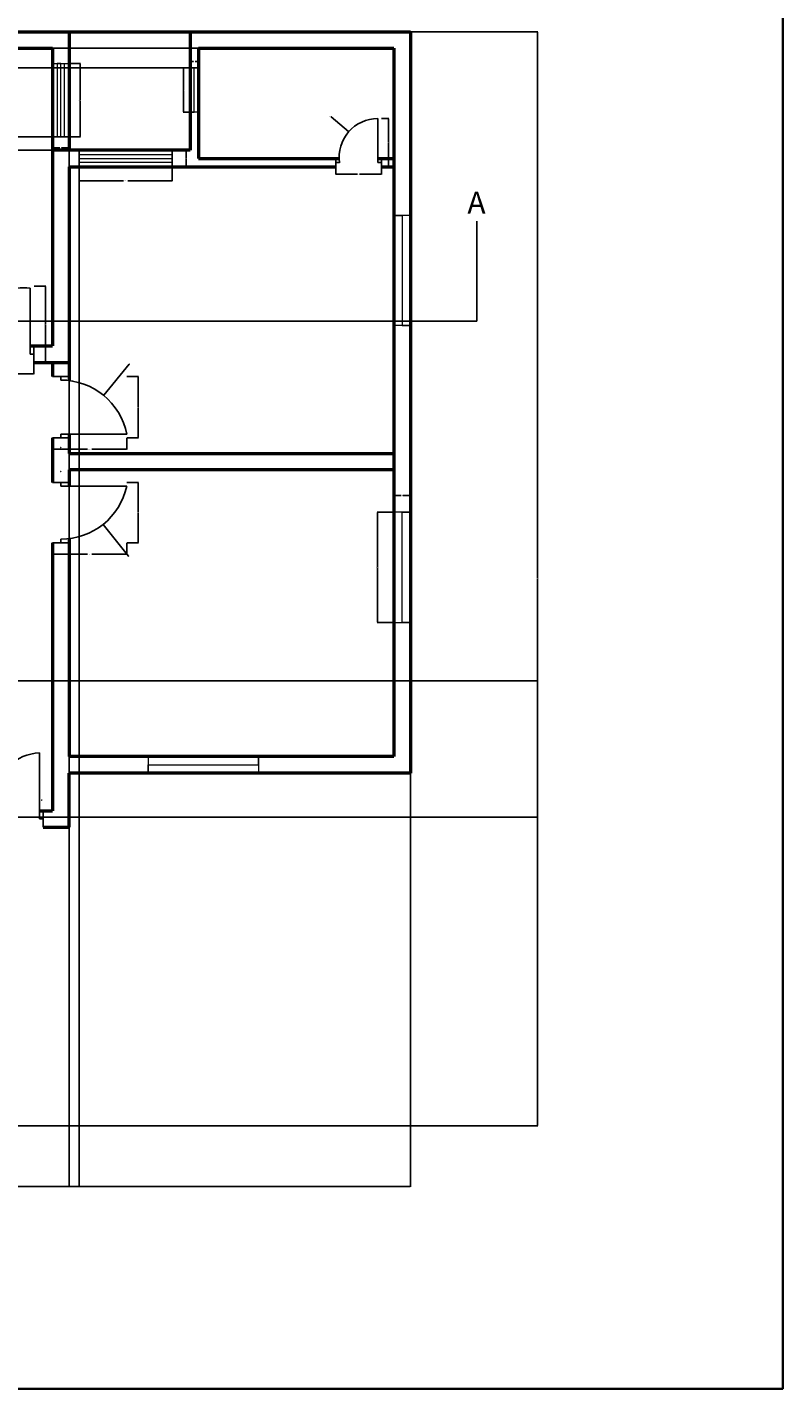
# Model space of a CAD drawing. Units: inches. Extents: x 2215 to 3724, y 1009 to 2124.
# Tile 10 of 11: x 3312 to 3724, y 1009 to 1750. Entities that reach past the tile are written whole.
import ezdxf

# ---------------------------------------------------------------- set-up
doc = ezdxf.new("R2010")
doc.units = ezdxf.units.IN
for name, color, linetype, lineweight in [('A-ANNO-DIMS', 2, 'Continuous', 18), ('A-ANNO-SYMB', 7, 'Continuous', 25), ('A-ANNO-TTLB', 7, 'Continuous', 35), ('A-DOOR', 3, 'Continuous', 25), ('A-GLAZ', 4, 'Continuous', 18), ('A-WALL', 7, 'Continuous', 50)]:
    doc.layers.add(name, color=color, linetype=linetype, lineweight=lineweight)
doc.styles.get("Standard").update_dxf_attribs({"font": 'arial.ttf'})
doc.dimstyles.get("Standard").update_dxf_attribs({"dimtxt": 0.18, "dimasz": 0.18, "dimexe": 0.18, "dimexo": 0.0625, "dimgap": 0.09, "dimtad": 0, "dimtih": 1, "dimtoh": 1, "dimdec": 4, "dimzin": 0, "dimdsep": 46, "dimtxsty": 'Standard', "dimcen": 0.09, "dimadec": 0, "dimazin": 0, "dimtfac": 1, "dimtdec": 4, "dimtofl": 0, "dimtmove": 0, "dimatfit": 3, "dimfxl": 1, "dimtolj": 1, "dimtzin": 0, "dimarcsym": 0})

# ---------------------------------------------------------------- blocks, each defined once
blk = doc.blocks.new('DOOR-BEDROOM-NE')
for p, q in [((0, 33.52), (0, 33.52)), ((0, 33.52), (9, 33.52)), ((9, 33.52), (4.5, 33.52)), ((4.5, 33.52), (4.5, 31.52)), ((0, 0), (9, 0)), ((4.5, 0), (4.5, 2)), ((4.5, 2), (40.5, 2)), ((9, 0), (4.5, 0))]:
    blk.add_line(p, q)
blk.add_arc((4.5, -5.19), 36.71, 11.299, 90)
blk = doc.blocks.new('DOOR-BEDROOM-SE')
for p, q in [((9, 32.82), (0, 32.82)), ((0, 32.82), (4.5, 32.82)), ((4.5, 32.82), (4.5, 30.82)), ((4.5, 30.82), (40.5, 30.82)), ((0, 0), (0, 0)), ((0, 0), (9, 0)), ((4.5, 0), (4.5, 2)), ((9, 0), (4.5, 0))]:
    blk.add_line(p, q)
blk.add_arc((4.5, 38.9), 36.9, 270, 347.35338)
blk = doc.blocks.new('DOOR-ENTRY-PAIR')
for p, q in [((2, 4.5), (2, 40.5)), ((54.26, 4.5), (54.26, 40.5)), ((0, 9), (0, 0)), ((56.26, 9), (56.26, 0)), ((0, 0), (0, 4.5)), ((0, 4.5), (2, 4.5)), ((56.26, 4.5), (54.26, 4.5))]:
    blk.add_line(p, q)
for centre, radius, start, end in [((2, 12.02), 28.48, 11.01665, 90), ((55.55, 14.8), 25.73, 92.87958, 174.07084)]:
    blk.add_arc(centre, radius, start, end)
blk = doc.blocks.new('DOOR-BATH-NE')
for p, q in [((22.84, 2.25), (22.84, 26.25)), ((0, 4.5), (0, 0)), ((0, 0), (0, 2.25)), ((0, 2.25), (2, 2.25)), ((24.84, 2.25), (22.84, 2.25)), ((24.84, 4.5), (24.84, 0)), ((24.84, 0), (24.84, 2.25))]:
    blk.add_line(p, q)
blk.add_arc((22.84, 5.2), 21.05, 90, 188.0713)
blk = doc.blocks.new('DOOR-BEDROOM-N')
for p, q in [((37.14, 4.5), (37.14, 40.5)), ((0, 9), (0, 0)), ((39.14, 9), (39.14, 0)), ((0, 0), (0, 4.5)), ((0, 4.5), (2, 4.5)), ((39.14, 4.5), (37.14, 4.5)), ((39.14, 0), (39.14, 4.5))]:
    blk.add_line(p, q)
blk.add_arc((33.66, 8.74), 31.95, 83.74408, 187.63495)
blk = doc.blocks.new('WIN-60-JAMB-A')
for p, q in [((0, 9), (0, 0)), ((60, 4.5), (60, 9)), ((60, 9), (60, 0)), ((0, 0), (0, 4.5)), ((0, 4.5), (60, 4.5))]:
    blk.add_line(p, q)
blk = doc.blocks.new('WIN-OTS-E-END')
for p, q in [((0, 9), (0, 0)), ((50.62, 4.5), (50.62, 9)), ((50.62, 9), (50.62, 0)), ((50.62, 6.5), (0, 6.5)), ((0, 6.5), (0, 4.5)), ((0, 0), (0, 4.5)), ((0, 4.5), (50.62, 4.5)), ((0, 4.5), (0, 2.5)), ((0, 2.5), (50.62, 2.5)), ((50.62, 4.5), (50.62, 6.5)), ((50.62, 0), (50.62, 4.5))]:
    blk.add_line(p, q)
blk = doc.blocks.new('WIN-60-JAMB-B')
for p, q in [((9, 60), (0, 60)), ((0, 60), (4.5, 60)), ((4.5, 60), (4.5, 0)), ((4.5, 0), (0, 0)), ((0, 0), (9, 0))]:
    blk.add_line(p, q)
blk = doc.blocks.new('WIN-OTS-E-SIDE')
for p, q in [((0, 39.84), (9, 39.84)), ((3.5, 39.84), (2.5, 39.84)), ((2.5, 39.84), (2.5, 0)), ((4.5, 39.84), (3.5, 39.84)), ((4.5, 0), (4.5, 39.84)), ((6.5, 0), (6.5, 39.84)), ((9, 0), (0, 0)), ((0, 0), (4.5, 0)), ((2.5, 0), (4.5, 0)), ((4.5, 0), (6.5, 0))]:
    blk.add_line(p, q)
blk = doc.blocks.new('VENT-24-NE')
for p, q in [((0, 24), (4.5, 24)), ((4.5, 24), (2.25, 24)), ((2.25, 24), (2.25, 0)), ((2.25, 0), (0, 0)), ((0, 0), (4.5, 0))]:
    blk.add_line(p, q)
blk = doc.blocks.new('*D33')
at = {"layer": 'A-ANNO-DIMS', "color": 0, "lineweight": -2, "transparency": 16777216}
for p, q in [((3511.68, 1485.98), (3502.56, 1485.98)), ((3502.74, 1485.8), (3502.74, 1456.16)), ((3502.74, 1426.16), (3502.74, 1455.79)), ((3511.68, 1425.98), (3502.56, 1425.98))]:
    blk.add_line(p, q, dxfattribs=at)
at = {"layer": 'A-ANNO-DIMS', "color": 0, "transparency": 16777216}
for points in [[(3502.71, 1485.8), (3502.77, 1485.8), (3502.74, 1485.98)], [(3502.71, 1426.16), (3502.77, 1426.16), (3502.74, 1425.98)]]:
    blk.add_solid(points, dxfattribs=at)
at = {"layer": 'Defpoints', "color": 0, "transparency": 16777216}
for p in [(3511.74, 1485.98), (3502.74, 1425.98), (3511.74, 1425.98)]:
    blk.add_point(p, dxfattribs=at)
at = {"layer": 'A-ANNO-DIMS', "color": 0, "transparency": 16777216, "insert": (3502.74, 1455.98), "char_height": 0.18, "attachment_point": 5}
blk.add_mtext('\\A1;WINDOW 60 TYP.', dxfattribs=at)
blk = doc.blocks.new('*D34')
at = {"layer": 'A-ANNO-DIMS', "color": 0, "lineweight": -2, "transparency": 16777216}
for p, q in [((3511.74, 1486.04), (3511.74, 1495.16)), ((3511.92, 1494.98), (3515.79, 1494.98)), ((3520.56, 1494.98), (3516.7, 1494.98)), ((3520.74, 1486.04), (3520.74, 1495.16))]:
    blk.add_line(p, q, dxfattribs=at)
at = {"layer": 'A-ANNO-DIMS', "color": 0, "transparency": 16777216}
for points in [[(3511.92, 1495.01), (3511.92, 1494.95), (3511.74, 1494.98)], [(3520.56, 1495.01), (3520.56, 1494.95), (3520.74, 1494.98)]]:
    blk.add_solid(points, dxfattribs=at)
at = {"layer": 'Defpoints', "color": 0, "transparency": 16777216}
for p in [(3511.74, 1494.98), (3511.74, 1485.98), (3520.74, 1485.98)]:
    blk.add_point(p, dxfattribs=at)
at = {"layer": 'A-ANNO-DIMS', "color": 0, "transparency": 16777216, "insert": (3516.24, 1494.98), "char_height": 0.18, "attachment_point": 5}
blk.add_mtext('\\A1;9 TYP.', dxfattribs=at)
blk = doc.blocks.new('*D35')
at = {"layer": 'A-ANNO-DIMS', "color": 0, "lineweight": -2, "transparency": 16777216}
for p, q in [((3340.3, 1673.93), (3340.3, 1666.22)), ((3390.92, 1673.93), (3390.92, 1666.22)), ((3340.48, 1666.4), (3364.49, 1666.4)), ((3390.74, 1666.4), (3366.73, 1666.4))]:
    blk.add_line(p, q, dxfattribs=at)
at = {"layer": 'A-ANNO-DIMS', "color": 0, "transparency": 16777216}
for points in [[(3340.48, 1666.43), (3340.48, 1666.37), (3340.3, 1666.4)], [(3390.74, 1666.43), (3390.74, 1666.37), (3390.92, 1666.4)]]:
    blk.add_solid(points, dxfattribs=at)
at = {"layer": 'Defpoints', "color": 0, "transparency": 16777216}
for p in [(3340.3, 1674), (3390.92, 1674), (3390.92, 1666.4)]:
    blk.add_point(p, dxfattribs=at)
at = {"layer": 'A-ANNO-DIMS', "color": 0, "transparency": 16777216, "insert": (3365.61, 1666.4), "char_height": 0.18, "attachment_point": 5}
blk.add_mtext('\\A1;WINDOW 51 TYP.', dxfattribs=at)
blk = doc.blocks.new('*D36')
at = {"layer": 'A-ANNO-DIMS', "color": 0, "lineweight": -2, "transparency": 16777216}
for p, q in [((3390.98, 1683), (3398.69, 1683)), ((3398.51, 1682.82), (3398.51, 1678.68)), ((3398.51, 1674.18), (3398.51, 1678.32)), ((3390.98, 1674), (3398.69, 1674))]:
    blk.add_line(p, q, dxfattribs=at)
at = {"layer": 'A-ANNO-DIMS', "color": 0, "transparency": 16777216}
for points in [[(3398.48, 1682.82), (3398.54, 1682.82), (3398.51, 1683)], [(3398.48, 1674.18), (3398.54, 1674.18), (3398.51, 1674)]]:
    blk.add_solid(points, dxfattribs=at)
at = {"layer": 'Defpoints', "color": 0, "transparency": 16777216}
for p in [(3390.92, 1683), (3398.51, 1683), (3390.92, 1674)]:
    blk.add_point(p, dxfattribs=at)
at = {"layer": 'A-ANNO-DIMS', "color": 0, "transparency": 16777216, "insert": (3398.51, 1678.5), "char_height": 0.18, "attachment_point": 5}
blk.add_mtext('\\A1;9 TYP.', dxfattribs=at)
blk = doc.blocks.new('*D37')
at = {"layer": 'A-ANNO-DIMS', "color": 0, "lineweight": -2, "transparency": 16777216}
for p, q in [((3334.81, 1730.15), (3340.9, 1730.15)), ((3340.72, 1729.97), (3340.72, 1710.41)), ((3340.72, 1690.49), (3340.72, 1710.05)), ((3334.81, 1690.31), (3340.9, 1690.31))]:
    blk.add_line(p, q, dxfattribs=at)
at = {"layer": 'A-ANNO-DIMS', "color": 0, "transparency": 16777216}
for points in [[(3340.69, 1729.97), (3340.75, 1729.97), (3340.72, 1730.15)], [(3340.69, 1690.49), (3340.75, 1690.49), (3340.72, 1690.31)]]:
    blk.add_solid(points, dxfattribs=at)
at = {"layer": 'Defpoints', "color": 0, "transparency": 16777216}
for p in [(3334.74, 1730.15), (3340.72, 1730.15), (3334.74, 1690.31)]:
    blk.add_point(p, dxfattribs=at)
at = {"layer": 'A-ANNO-DIMS', "color": 0, "transparency": 16777216, "insert": (3340.72, 1710.23), "char_height": 0.18, "attachment_point": 5}
blk.add_mtext('\\A1;WINDOW 40 TYP.', dxfattribs=at)
blk = doc.blocks.new('*D38')
at = {"layer": 'A-ANNO-DIMS', "color": 0, "lineweight": -2, "transparency": 16777216}
for p, q in [((3325.74, 1690.25), (3325.74, 1684.15)), ((3334.74, 1690.25), (3334.74, 1684.15)), ((3325.92, 1684.33), (3329.79, 1684.33)), ((3334.56, 1684.33), (3330.7, 1684.33))]:
    blk.add_line(p, q, dxfattribs=at)
at = {"layer": 'A-ANNO-DIMS', "color": 0, "transparency": 16777216}
for points in [[(3325.92, 1684.36), (3325.92, 1684.3), (3325.74, 1684.33)], [(3334.56, 1684.36), (3334.56, 1684.3), (3334.74, 1684.33)]]:
    blk.add_solid(points, dxfattribs=at)
at = {"layer": 'Defpoints', "color": 0, "transparency": 16777216}
for p in [(3325.74, 1690.31), (3334.74, 1690.31), (3334.74, 1684.33)]:
    blk.add_point(p, dxfattribs=at)
at = {"layer": 'A-ANNO-DIMS', "color": 0, "transparency": 16777216, "insert": (3330.24, 1684.33), "char_height": 0.18, "attachment_point": 5}
blk.add_mtext('\\A1;9 TYP.', dxfattribs=at)
blk = doc.blocks.new('*D49')
at = {"layer": 'A-ANNO-DIMS', "color": 0, "lineweight": -2, "transparency": 16777216}
for p, q in [((3400.68, 1727.79), (3396.96, 1727.79)), ((3397.14, 1727.61), (3397.14, 1715.97)), ((3397.14, 1703.97), (3397.14, 1715.61)), ((3400.68, 1703.79), (3396.96, 1703.79))]:
    blk.add_line(p, q, dxfattribs=at)
at = {"layer": 'A-ANNO-DIMS', "color": 0, "transparency": 16777216}
for points in [[(3397.11, 1727.61), (3397.17, 1727.61), (3397.14, 1727.79)], [(3397.11, 1703.97), (3397.17, 1703.97), (3397.14, 1703.79)]]:
    blk.add_solid(points, dxfattribs=at)
at = {"layer": 'Defpoints', "color": 0, "transparency": 16777216}
for p in [(3400.74, 1727.79), (3397.14, 1703.79), (3400.74, 1703.79)]:
    blk.add_point(p, dxfattribs=at)
at = {"layer": 'A-ANNO-DIMS', "color": 0, "transparency": 16777216, "insert": (3397.14, 1715.79), "char_height": 0.18, "attachment_point": 5}
blk.add_mtext('\\A1;VENT 24 TYP.', dxfattribs=at)
blk = doc.blocks.new('*D50')
at = {"layer": 'A-ANNO-DIMS', "color": 0, "lineweight": -2, "transparency": 16777216}
for p, q in [((3400.74, 1727.85), (3400.74, 1731.57)), ((3400.92, 1731.39), (3402.54, 1731.39)), ((3405.06, 1731.39), (3403.45, 1731.39)), ((3405.24, 1727.85), (3405.24, 1731.57))]:
    blk.add_line(p, q, dxfattribs=at)
at = {"layer": 'A-ANNO-DIMS', "color": 0, "transparency": 16777216}
for points in [[(3400.92, 1731.42), (3400.92, 1731.36), (3400.74, 1731.39)], [(3405.06, 1731.42), (3405.06, 1731.36), (3405.24, 1731.39)]]:
    blk.add_solid(points, dxfattribs=at)
at = {"layer": 'Defpoints', "color": 0, "transparency": 16777216}
for p in [(3400.74, 1731.39), (3400.74, 1727.79), (3405.24, 1727.79)]:
    blk.add_point(p, dxfattribs=at)
at = {"layer": 'A-ANNO-DIMS', "color": 0, "transparency": 16777216, "insert": (3402.99, 1731.39), "char_height": 0.18, "attachment_point": 5}
blk.add_mtext('\\A1;5 TYP.', dxfattribs=at)
blk = doc.blocks.new('*D53')
at = {"layer": 'A-ANNO-DIMS', "color": 0, "lineweight": -2, "transparency": 16777216}
for p, q in [((3325.74, 1526.33), (3325.74, 1520.14)), ((3325.92, 1520.32), (3344.85, 1520.32)), ((3366.06, 1520.32), (3347.14, 1520.32)), ((3366.24, 1526.33), (3366.24, 1520.14))]:
    blk.add_line(p, q, dxfattribs=at)
at = {"layer": 'A-ANNO-DIMS', "color": 0, "transparency": 16777216}
for points in [[(3325.92, 1520.35), (3325.92, 1520.29), (3325.74, 1520.32)], [(3366.06, 1520.35), (3366.06, 1520.29), (3366.24, 1520.32)]]:
    blk.add_solid(points, dxfattribs=at)
at = {"layer": 'Defpoints', "color": 0, "transparency": 16777216}
for p in [(3325.74, 1526.4), (3366.24, 1526.4), (3366.24, 1520.32)]:
    blk.add_point(p, dxfattribs=at)
at = {"layer": 'A-ANNO-DIMS', "color": 0, "transparency": 16777216, "insert": (3345.99, 1520.32), "char_height": 0.18, "attachment_point": 5}
blk.add_mtext('\\A1;BR DOOR 41 TYP.', dxfattribs=at)
blk = doc.blocks.new('*D54')
at = {"layer": 'A-ANNO-DIMS', "color": 0, "lineweight": -2, "transparency": 16777216}
for p, q in [((3366.31, 1559.91), (3372.5, 1559.91)), ((3372.32, 1559.73), (3372.32, 1543.34)), ((3372.32, 1526.58), (3372.32, 1542.97)), ((3366.31, 1526.4), (3372.5, 1526.4))]:
    blk.add_line(p, q, dxfattribs=at)
at = {"layer": 'A-ANNO-DIMS', "color": 0, "transparency": 16777216}
for points in [[(3372.29, 1559.73), (3372.35, 1559.73), (3372.32, 1559.91)], [(3372.29, 1526.58), (3372.35, 1526.58), (3372.32, 1526.4)]]:
    blk.add_solid(points, dxfattribs=at)
at = {"layer": 'Defpoints', "color": 0, "transparency": 16777216}
for p in [(3366.24, 1559.91), (3372.32, 1559.91), (3366.24, 1526.4)]:
    blk.add_point(p, dxfattribs=at)
at = {"layer": 'A-ANNO-DIMS', "color": 0, "transparency": 16777216, "insert": (3372.32, 1543.15), "char_height": 0.18, "attachment_point": 5}
blk.add_mtext('\\A1;34 TYP.', dxfattribs=at)
blk = doc.blocks.new('*D55')
at = {"layer": 'A-ANNO-DIMS', "color": 0, "lineweight": -2, "transparency": 16777216}
for p, q in [((3325.74, 1469.19), (3325.74, 1463)), ((3366.24, 1469.19), (3366.24, 1463)), ((3325.92, 1463.18), (3344.85, 1463.18)), ((3366.06, 1463.18), (3347.14, 1463.18))]:
    blk.add_line(p, q, dxfattribs=at)
at = {"layer": 'A-ANNO-DIMS', "color": 0, "transparency": 16777216}
for points in [[(3325.92, 1463.21), (3325.92, 1463.15), (3325.74, 1463.18)], [(3366.06, 1463.21), (3366.06, 1463.15), (3366.24, 1463.18)]]:
    blk.add_solid(points, dxfattribs=at)
at = {"layer": 'Defpoints', "color": 0, "transparency": 16777216}
for p in [(3325.74, 1469.26), (3366.24, 1469.26), (3366.24, 1463.18)]:
    blk.add_point(p, dxfattribs=at)
at = {"layer": 'A-ANNO-DIMS', "color": 0, "transparency": 16777216, "insert": (3345.99, 1463.18), "char_height": 0.18, "attachment_point": 5}
blk.add_mtext('\\A1;BR DOOR 41 TYP.', dxfattribs=at)
blk = doc.blocks.new('*D56')
at = {"layer": 'A-ANNO-DIMS', "color": 0, "lineweight": -2, "transparency": 16777216}
for p, q in [((3366.31, 1502.07), (3372.5, 1502.07)), ((3372.32, 1501.89), (3372.32, 1485.85)), ((3372.32, 1469.44), (3372.32, 1485.48)), ((3366.31, 1469.26), (3372.5, 1469.26))]:
    blk.add_line(p, q, dxfattribs=at)
at = {"layer": 'A-ANNO-DIMS', "color": 0, "transparency": 16777216}
for points in [[(3372.29, 1501.89), (3372.35, 1501.89), (3372.32, 1502.07)], [(3372.29, 1469.44), (3372.35, 1469.44), (3372.32, 1469.26)]]:
    blk.add_solid(points, dxfattribs=at)
at = {"layer": 'Defpoints', "color": 0, "transparency": 16777216}
for p in [(3366.24, 1502.07), (3372.32, 1502.07), (3366.24, 1469.26)]:
    blk.add_point(p, dxfattribs=at)
at = {"layer": 'A-ANNO-DIMS', "color": 0, "transparency": 16777216, "insert": (3372.32, 1485.67), "char_height": 0.18, "attachment_point": 5}
blk.add_mtext('\\A1;33 TYP.', dxfattribs=at)
blk = doc.blocks.new('*D59')
at = {"layer": 'A-ANNO-DIMS', "color": 0, "lineweight": -2, "transparency": 16777216}
for p, q in [((3505.02, 1700.25), (3509.07, 1700.25)), ((3508.89, 1700.07), (3508.89, 1687.31)), ((3508.89, 1674.18), (3508.89, 1686.94)), ((3505.02, 1674), (3509.07, 1674))]:
    blk.add_line(p, q, dxfattribs=at)
at = {"layer": 'A-ANNO-DIMS', "color": 0, "transparency": 16777216}
for points in [[(3508.86, 1700.07), (3508.92, 1700.07), (3508.89, 1700.25)], [(3508.86, 1674.18), (3508.92, 1674.18), (3508.89, 1674)]]:
    blk.add_solid(points, dxfattribs=at)
at = {"layer": 'Defpoints', "color": 0, "transparency": 16777216}
for p in [(3504.95, 1700.25), (3508.89, 1700.25), (3504.95, 1674)]:
    blk.add_point(p, dxfattribs=at)
at = {"layer": 'A-ANNO-DIMS', "color": 0, "transparency": 16777216, "insert": (3508.89, 1687.12), "char_height": 0.18, "attachment_point": 5}
blk.add_mtext('\\A1;WC DOOR 26 TYP.', dxfattribs=at)
blk = doc.blocks.new('*D60')
at = {"layer": 'A-ANNO-DIMS', "color": 0, "lineweight": -2, "transparency": 16777216}
for p, q in [((3480.12, 1673.93), (3480.12, 1669.88)), ((3480.3, 1670.06), (3492.01, 1670.06)), ((3504.77, 1670.06), (3493.07, 1670.06)), ((3504.95, 1673.93), (3504.95, 1669.88))]:
    blk.add_line(p, q, dxfattribs=at)
at = {"layer": 'A-ANNO-DIMS', "color": 0, "transparency": 16777216}
for points in [[(3480.3, 1670.09), (3480.3, 1670.03), (3480.12, 1670.06)], [(3504.77, 1670.09), (3504.77, 1670.03), (3504.95, 1670.06)]]:
    blk.add_solid(points, dxfattribs=at)
at = {"layer": 'Defpoints', "color": 0, "transparency": 16777216}
for p in [(3480.12, 1674), (3504.95, 1674), (3504.95, 1670.06)]:
    blk.add_point(p, dxfattribs=at)
at = {"layer": 'A-ANNO-DIMS', "color": 0, "transparency": 16777216, "insert": (3492.54, 1670.06), "char_height": 0.18, "attachment_point": 5}
blk.add_mtext('\\A1;25 TYP.', dxfattribs=at)
blk = doc.blocks.new('*D61')
at = {"layer": 'A-ANNO-DIMS', "color": 0, "lineweight": -2, "transparency": 16777216}
for p, q in [((3315.7, 1609.07), (3322.06, 1609.07)), ((3321.88, 1608.89), (3321.88, 1588.47)), ((3321.88, 1567.68), (3321.88, 1588.1)), ((3315.7, 1567.5), (3322.06, 1567.5))]:
    blk.add_line(p, q, dxfattribs=at)
at = {"layer": 'A-ANNO-DIMS', "color": 0, "transparency": 16777216}
for points in [[(3321.85, 1608.89), (3321.91, 1608.89), (3321.88, 1609.07)], [(3321.85, 1567.68), (3321.91, 1567.68), (3321.88, 1567.5)]]:
    blk.add_solid(points, dxfattribs=at)
at = {"layer": 'Defpoints', "color": 0, "transparency": 16777216}
for p in [(3315.64, 1609.07), (3321.88, 1609.07), (3315.64, 1567.5)]:
    blk.add_point(p, dxfattribs=at)
at = {"layer": 'A-ANNO-DIMS', "color": 0, "transparency": 16777216, "insert": (3321.88, 1588.28), "char_height": 0.18, "attachment_point": 5}
blk.add_mtext('\\A1;BR DOOR 42 TYP.', dxfattribs=at)
blk = doc.blocks.new('*D62')
at = {"layer": 'A-ANNO-DIMS', "color": 0, "lineweight": -2, "transparency": 16777216}
for p, q in [((3276.5, 1567.43), (3276.5, 1561.08)), ((3315.64, 1567.43), (3315.64, 1561.08)), ((3276.68, 1561.26), (3295.54, 1561.26)), ((3315.46, 1561.26), (3296.6, 1561.26))]:
    blk.add_line(p, q, dxfattribs=at)
at = {"layer": 'A-ANNO-DIMS', "color": 0, "transparency": 16777216}
for points in [[(3276.68, 1561.29), (3276.68, 1561.23), (3276.5, 1561.26)], [(3315.46, 1561.29), (3315.46, 1561.23), (3315.64, 1561.26)]]:
    blk.add_solid(points, dxfattribs=at)
at = {"layer": 'Defpoints', "color": 0, "transparency": 16777216}
for p in [(3276.5, 1567.5), (3315.64, 1567.5), (3315.64, 1561.26)]:
    blk.add_point(p, dxfattribs=at)
at = {"layer": 'A-ANNO-DIMS', "color": 0, "transparency": 16777216, "insert": (3296.07, 1561.26), "char_height": 0.18, "attachment_point": 5}
blk.add_mtext('\\A1;39 TYP.', dxfattribs=at)
blk = doc.blocks.new('*D96')
at = {"layer": 'A-ANNO-DIMS', "color": 0, "lineweight": -2, "transparency": 16777216}
for p, q in [((3520.74, 1343.93), (3520.74, 1118.67)), ((2962.74, 1151.93), (2962.74, 1118.67)), ((2962.92, 1118.85), (3241.45, 1118.85)), ((3520.56, 1118.85), (3242.03, 1118.85))]:
    blk.add_line(p, q, dxfattribs=at)
at = {"layer": 'A-ANNO-DIMS', "color": 0, "transparency": 16777216}
for points in [[(2962.92, 1118.88), (2962.92, 1118.82), (2962.74, 1118.85)], [(3520.56, 1118.88), (3520.56, 1118.82), (3520.74, 1118.85)]]:
    blk.add_solid(points, dxfattribs=at)
at = {"layer": 'Defpoints', "color": 0, "transparency": 16777216}
for p in [(3520.74, 1344), (2962.74, 1152), (3520.74, 1118.85)]:
    blk.add_point(p, dxfattribs=at)
at = {"layer": 'A-ANNO-DIMS', "color": 0, "transparency": 16777216, "insert": (3241.74, 1118.85), "char_height": 0.18, "attachment_point": 5}
blk.add_mtext('\\A1;558', dxfattribs=at)
blk = doc.blocks.new('*D97')
at = {"layer": 'A-ANNO-DIMS', "color": 0, "lineweight": -2, "transparency": 16777216}
for p, q in [((3520.81, 1747.5), (3590.27, 1747.5)), ((3590.09, 1747.32), (3590.09, 1449.93)), ((3590.09, 1152.18), (3590.09, 1449.57)), ((3259.81, 1152), (3590.27, 1152))]:
    blk.add_line(p, q, dxfattribs=at)
at = {"layer": 'A-ANNO-DIMS', "color": 0, "transparency": 16777216}
for points in [[(3590.06, 1747.32), (3590.12, 1747.32), (3590.09, 1747.5)], [(3590.06, 1152.18), (3590.12, 1152.18), (3590.09, 1152)]]:
    blk.add_solid(points, dxfattribs=at)
at = {"layer": 'Defpoints', "color": 0, "transparency": 16777216}
for p in [(3520.74, 1747.5), (3590.09, 1747.5), (3259.74, 1152)]:
    blk.add_point(p, dxfattribs=at)
at = {"layer": 'A-ANNO-DIMS', "color": 0, "transparency": 16777216, "insert": (3590.09, 1449.75), "char_height": 0.18, "attachment_point": 5}
blk.add_mtext('\\A1;595.5', dxfattribs=at)
blk = doc.blocks.new('*D123')
at = {"layer": 'A-ANNO-DIMS', "color": 0, "lineweight": -2, "transparency": 16777216}
for p, q in [((3334.74, 1682.93), (3334.74, 1118.67)), ((3340.3, 1682.93), (3340.3, 1118.67)), ((3334.92, 1118.85), (3337.13, 1118.85)), ((3340.12, 1118.85), (3337.92, 1118.85))]:
    blk.add_line(p, q, dxfattribs=at)
at = {"layer": 'A-ANNO-DIMS', "color": 0, "transparency": 16777216}
for points in [[(3334.92, 1118.88), (3334.92, 1118.82), (3334.74, 1118.85)], [(3340.12, 1118.88), (3340.12, 1118.82), (3340.3, 1118.85)]]:
    blk.add_solid(points, dxfattribs=at)
at = {"layer": 'Defpoints', "color": 0, "transparency": 16777216}
for p in [(3334.74, 1683), (3340.3, 1683), (3340.3, 1118.85)]:
    blk.add_point(p, dxfattribs=at)
at = {"layer": 'A-ANNO-DIMS', "color": 0, "transparency": 16777216, "insert": (3337.52, 1118.85), "char_height": 0.18, "attachment_point": 5}
blk.add_mtext('\\A1;5.558', dxfattribs=at)
blk = doc.blocks.new('*D124')
at = {"layer": 'A-ANNO-DIMS', "color": 0, "lineweight": -2, "transparency": 16777216}
for p, q in [((3334.68, 1690.31), (2877.61, 1690.31)), ((2877.79, 1690.13), (2877.79, 1686.83)), ((3334.68, 1683), (2877.61, 1683)), ((2877.79, 1683.18), (2877.79, 1686.47))]:
    blk.add_line(p, q, dxfattribs=at)
at = {"layer": 'A-ANNO-DIMS', "color": 0, "transparency": 16777216}
for points in [[(2877.76, 1690.13), (2877.82, 1690.13), (2877.79, 1690.31)], [(2877.76, 1683.18), (2877.82, 1683.18), (2877.79, 1683)]]:
    blk.add_solid(points, dxfattribs=at)
at = {"layer": 'Defpoints', "color": 0, "transparency": 16777216}
for p in [(2877.79, 1690.31), (3334.74, 1690.31), (3334.74, 1683)]:
    blk.add_point(p, dxfattribs=at)
at = {"layer": 'A-ANNO-DIMS', "color": 0, "transparency": 16777216, "insert": (2877.79, 1686.65), "char_height": 0.18, "attachment_point": 5}
blk.add_mtext('\\A1;7.31', dxfattribs=at)
blk = doc.blocks.new('*D125')
at = {"layer": 'A-ANNO-DIMS', "color": 0, "lineweight": -2, "transparency": 16777216}
for p, q in [((3405.18, 1738.5), (2877.61, 1738.5)), ((2877.79, 1738.32), (2877.79, 1733.33)), ((3405.18, 1727.79), (2877.61, 1727.79)), ((2877.79, 1727.97), (2877.79, 1732.96))]:
    blk.add_line(p, q, dxfattribs=at)
at = {"layer": 'A-ANNO-DIMS', "color": 0, "transparency": 16777216}
for points in [[(2877.76, 1738.32), (2877.82, 1738.32), (2877.79, 1738.5)], [(2877.76, 1727.97), (2877.82, 1727.97), (2877.79, 1727.79)]]:
    blk.add_solid(points, dxfattribs=at)
at = {"layer": 'Defpoints', "color": 0, "transparency": 16777216}
for p in [(2877.79, 1738.5), (3405.24, 1738.5), (3405.24, 1727.79)]:
    blk.add_point(p, dxfattribs=at)
at = {"layer": 'A-ANNO-DIMS', "color": 0, "transparency": 16777216, "insert": (2877.79, 1733.14), "char_height": 0.18, "attachment_point": 5}
blk.add_mtext('\\A1;10.706', dxfattribs=at)
blk = doc.blocks.new('*D128')
at = {"layer": 'A-ANNO-DIMS', "color": 0, "lineweight": -2, "transparency": 16777216}
for p, q in [((3075.31, 1394.25), (3590.27, 1394.25)), ((3590.09, 1394.07), (3590.09, 1357.31)), ((3590.09, 1320.18), (3590.09, 1356.94)), ((3075.31, 1320), (3590.27, 1320))]:
    blk.add_line(p, q, dxfattribs=at)
at = {"layer": 'A-ANNO-DIMS', "color": 0, "transparency": 16777216}
for points in [[(3590.06, 1394.07), (3590.12, 1394.07), (3590.09, 1394.25)], [(3590.06, 1320.18), (3590.12, 1320.18), (3590.09, 1320)]]:
    blk.add_solid(points, dxfattribs=at)
at = {"layer": 'Defpoints', "color": 0, "transparency": 16777216}
for p in [(3075.24, 1394.25), (3590.09, 1394.25), (3075.24, 1320)]:
    blk.add_point(p, dxfattribs=at)
at = {"layer": 'A-ANNO-DIMS', "color": 0, "transparency": 16777216, "insert": (3590.09, 1357.13), "char_height": 0.18, "attachment_point": 5}
blk.add_mtext('\\A1;74.26', dxfattribs=at)
blk = doc.blocks.new('*D130')
at = {"layer": 'A-ANNO-DIMS', "color": 0, "lineweight": -2, "transparency": 16777216}
for p, q in [((3330.15, 1508.15), (3330.33, 1508.15)), ((3330.24, 1508.06), (3330.24, 1508.24)), ((3367.13, 1462.07), (3353.41, 1479.21)), ((3367.31, 1462.07), (3367.13, 1462.07))]:
    blk.add_line(p, q, dxfattribs=at)
at = {"layer": 'A-ANNO-DIMS', "color": 0, "transparency": 16777216}
blk.add_solid([(3353.44, 1479.23), (3353.39, 1479.19), (3353.3, 1479.35)], dxfattribs=at)
at = {"layer": 'Defpoints', "color": 0, "transparency": 16777216}
for p in [(3330.24, 1508.15), (3353.3, 1479.35)]:
    blk.add_point(p, dxfattribs=at)
at = {"layer": 'A-ANNO-DIMS', "color": 0, "transparency": 16777216, "insert": (3367.86, 1462.07), "char_height": 0.18, "attachment_point": 5}
blk.add_mtext('\\A1;R36.895', dxfattribs=at)
blk = doc.blocks.new('*D131')
at = {"layer": 'A-ANNO-DIMS', "color": 0, "lineweight": -2, "transparency": 16777216}
for p, q in [((3367.49, 1566.62), (3353.63, 1549.73)), ((3367.67, 1566.62), (3367.49, 1566.62)), ((3330.15, 1521.2), (3330.33, 1521.2)), ((3330.24, 1521.11), (3330.24, 1521.29))]:
    blk.add_line(p, q, dxfattribs=at)
at = {"layer": 'A-ANNO-DIMS', "color": 0, "transparency": 16777216}
blk.add_solid([(3353.61, 1549.75), (3353.66, 1549.71), (3353.52, 1549.59)], dxfattribs=at)
at = {"layer": 'Defpoints', "color": 0, "transparency": 16777216}
for p in [(3353.52, 1549.59), (3330.24, 1521.2)]:
    blk.add_point(p, dxfattribs=at)
at = {"layer": 'A-ANNO-DIMS', "color": 0, "transparency": 16777216, "insert": (3368.13, 1566.62), "char_height": 0.18, "attachment_point": 5}
blk.add_mtext('\\A1;R36.71', dxfattribs=at)
blk = doc.blocks.new('*D138')
at = {"layer": 'A-ANNO-DIMS', "color": 0, "lineweight": -2, "transparency": 16777216}
for p, q in [((3291.4, 1359.16), (3291.58, 1359.16)), ((3291.58, 1359.16), (3302.08, 1348.09)), ((3319.82, 1329.29), (3320, 1329.29)), ((3319.91, 1329.2), (3319.91, 1329.38))]:
    blk.add_line(p, q, dxfattribs=at)
at = {"layer": 'A-ANNO-DIMS', "color": 0, "transparency": 16777216}
blk.add_solid([(3302.1, 1348.11), (3302.06, 1348.07), (3302.2, 1347.96)], dxfattribs=at)
at = {"layer": 'Defpoints', "color": 0, "transparency": 16777216}
for p in [(3302.2, 1347.96), (3319.91, 1329.29)]:
    blk.add_point(p, dxfattribs=at)
at = {"layer": 'A-ANNO-DIMS', "color": 0, "transparency": 16777216, "insert": (3290.92, 1359.16), "char_height": 0.18, "attachment_point": 5}
blk.add_mtext('\\A1;R25.73', dxfattribs=at)
blk = doc.blocks.new('*D140')
at = {"layer": 'A-ANNO-DIMS', "color": 0, "lineweight": -2, "transparency": 16777216}
for p, q in [((3477.35, 1701.28), (3477.53, 1701.28)), ((3477.53, 1701.28), (3486.93, 1693.12)), ((3502.86, 1679.2), (3503.04, 1679.2)), ((3502.95, 1679.11), (3502.95, 1679.29))]:
    blk.add_line(p, q, dxfattribs=at)
at = {"layer": 'A-ANNO-DIMS', "color": 0, "transparency": 16777216}
blk.add_solid([(3486.95, 1693.14), (3486.91, 1693.09), (3487.06, 1693)], dxfattribs=at)
at = {"layer": 'Defpoints', "color": 0, "transparency": 16777216}
for p in [(3487.06, 1693), (3502.95, 1679.2)]:
    blk.add_point(p, dxfattribs=at)
at = {"layer": 'A-ANNO-DIMS', "color": 0, "transparency": 16777216, "insert": (3476.8, 1701.28), "char_height": 0.18, "attachment_point": 5}
blk.add_mtext('\\A1;R21.045', dxfattribs=at)

msp = doc.modelspace()

# ---------------------------------------------------------------- linework, layer by layer
at = {"layer": 'A-ANNO-SYMB'}
for p, q in [((3556.9429, 1589.9969), (3556.9429, 1644.4569)), ((2910.9414, 1589.9969), (3556.9429, 1589.9969))]:
    msp.add_line(p, q, dxfattribs=at)
at = {"layer": 'A-ANNO-TTLB'}
msp.add_lwpolyline([(2215.4438, 2124.2681), (3723.6589, 2124.2681), (3723.6589, 1008.7935), (2215.4438, 1008.7935)], close=True, dxfattribs=at)
at = {"layer": 'A-WALL'}
for p, q in [((2962.7432, 1747.4969), (3520.7432, 1747.4969)), ((3334.7432, 1747.4969), (3334.7432, 1682.9969)), ((3400.7432, 1747.4969), (3400.7432, 1682.9969)), ((3520.7432, 1747.4969), (3520.7432, 1343.9969)), ((3157.7432, 1738.4969), (3325.7432, 1738.4969)), ((3325.7432, 1738.4969), (3325.7432, 1576.4969)), ((3405.2432, 1738.4969), (3405.2432, 1678.4969)), ((3405.2432, 1738.4969), (3511.7432, 1738.4969)), ((3511.7432, 1738.4969), (3511.7432, 1352.9969)), ((3334.7432, 1682.9969), (3325.7432, 1682.9969)), ((3400.7432, 1682.9969), (3334.7432, 1682.9969)), ((3405.2432, 1678.4969), (3481.9206, 1678.4969)), ((3502.954, 1678.4969), (3511.7432, 1678.4969)), ((3334.7432, 1673.9969), (3334.7432, 1567.4969)), ((3334.7432, 1673.9969), (3480.1173, 1673.9969)), ((3504.954, 1673.9969), (3511.7432, 1673.9969)), ((3313.6412, 1576.4969), (3325.7432, 1576.4969)), ((3313.6412, 1576.4969), (3325.7432, 1576.4969)), ((3313.6412, 1576.4969), (3325.7432, 1576.4969)), ((3315.6412, 1567.4969), (3334.7432, 1567.4969)), ((3325.7432, 1567.4969), (3325.7432, 1559.9139)), ((3334.7432, 1567.4969), (3334.7432, 1557.637)), ((3334.7432, 1528.3952), (3334.7432, 1517.9969)), ((3325.7432, 1526.3952), (3325.7432, 1502.0746)), ((3334.7432, 1517.9969), (3511.7432, 1517.9969)), ((3511.7432, 1508.9969), (3334.7432, 1508.9969)), ((3334.7432, 1508.9969), (3334.7432, 1500.0746)), ((3325.7432, 1469.2572), (3325.7432, 1343.9969)), ((3334.7432, 1471.5327), (3334.7432, 1352.9969)), ((3511.7432, 1352.9969), (3334.7432, 1352.9969)), ((3325.7432, 1343.9969), (3325.7432, 1323.4864)), ((3520.7432, 1343.9969), (3334.7432, 1343.9969)), ((3334.7432, 1318.9864), (3334.7432, 1343.9969)), ((3318.6141, 1323.4864), (3325.7432, 1323.4864)), ((3320.6141, 1314.4864), (3334.7432, 1314.4864)), ((3334.7432, 1314.4864), (3334.7432, 1318.9864))]:
    msp.add_line(p, q, dxfattribs=at)

# ---------------------------------------------------------------- block references
at = {"layer": 'A-DOOR'}
for name, p in [('DOOR-BATH-NE', (3480.1172, 1673.997)), ('DOOR-BEDROOM-N', (3276.4972, 1567.497)), ('DOOR-BEDROOM-NE', (3325.7432, 1526.395)), ('DOOR-BEDROOM-SE', (3325.7432, 1469.257)), ('DOOR-ENTRY-PAIR', (3264.3552, 1314.486))]:
    msp.add_blockref(name, p, dxfattribs=at)
at = {"layer": 'A-GLAZ'}
for name, p in [('WIN-OTS-E-SIDE', (3325.7432, 1690.308)), ('WIN-OTS-E-END', (3340.3012, 1673.997)), ('WIN-60-JAMB-A', (3377.8867, 1343.997))]:
    msp.add_blockref(name, p, dxfattribs=at)
for name, p, rotation in [('VENT-24-NE', (3405.2432, 1727.7909), 180), ('WIN-60-JAMB-A', (3511.7433, 1647.5401), 270.0000000000003), ('WIN-60-JAMB-B', (3520.7432, 1485.9762), 180)]:
    msp.add_blockref(name, p, dxfattribs=dict(at, rotation=rotation))

# ---------------------------------------------------------------- texts
at = {"layer": 'A-ANNO-SYMB', "insert": (3551.7885, 1660.4998), "char_height": 12, "attachment_point": 1}
msp.add_mtext_dynamic_manual_height_columns('A', width=26.651845, gutter_width=12.5, heights=[0], dxfattribs=at)

# ---------------------------------------------------------------- dimensions: what is measured, and where the dimension line sits
at = {"layer": 'A-ANNO-DIMS'}
for base, p1, p2, override, picture, middle in [((3590.0929, 1747.4969), (3259.7432, 1151.9969), (3520.7432, 1747.4969), {"dimdec": 1, "dimlfac": 1, "dimrnd": 0, "dimzin": 0, "dimdsep": 46, "dimlunit": 2}, '*D97', (3590.0929, 1449.7469)), ((2877.7914, 1738.4969), (3405.2432, 1727.7909), (3405.2432, 1738.4969), {"dimdec": 3, "dimlfac": 1, "dimrnd": 0, "dimzin": 0, "dimdsep": 46, "dimlunit": 2}, '*D125', (2877.7914, 1733.1439)), ((2877.7914, 1690.3077), (3334.7432, 1682.9969), (3334.7432, 1690.3077), {"dimdec": 2, "dimlfac": 1, "dimrnd": 0, "dimzin": 0, "dimdsep": 46, "dimlunit": 2}, '*D124', (2877.7914, 1686.6523)), ((3590.0929, 1394.2548), (3075.2432, 1319.9969), (3075.2432, 1394.2548), {"dimdec": 2, "dimlfac": 1, "dimrnd": 0, "dimzin": 0, "dimdsep": 46, "dimlunit": 2}, '*D128', (3590.0929, 1357.1259))]:
    dim = msp.add_linear_dim(base=base, p1=p1, p2=p2, angle=90, dimstyle='Standard', override=override, dxfattribs=at)
    dim.commit()
    dim.dimension.update_dxf_attribs({"geometry": picture, "text_midpoint": middle})
for base, p1, p2, angle, text, picture, middle in [((3340.7199, 1730.1526), (3334.7432, 1690.3077), (3334.7432, 1730.1526), 90, 'WINDOW <> TYP.', '*D37', (3340.7199, 1710.2302)), ((3397.1432, 1703.7909), (3400.7432, 1727.7909), (3400.7432, 1703.7909), 270, 'VENT <> TYP.', '*D49', (3397.1432, 1715.7909)), ((3400.7432030508, 1731.390947381), (3405.2432030508, 1727.790947381), (3400.7432030508, 1727.790947381), 180, '<> TYP.', '*D50', (3402.9932030508, 1731.390947381)), ((3508.8915, 1700.2469), (3504.954, 1673.9969), (3504.954, 1700.2469), 90, 'WC DOOR <> TYP.', '*D59', (3508.8915, 1687.1219)), ((3398.5085, 1682.9969), (3390.9163, 1673.9969), (3390.9163, 1682.9969), 90, '<> TYP.', '*D36', (3398.5085, 1678.4969)), ((3321.8767, 1609.0674), (3315.6412, 1567.4969), (3315.6412, 1609.0674), 90, 'BR DOOR <> TYP.', '*D61', (3321.8767, 1588.2821)), ((3372.3182, 1559.9139), (3366.2432, 1526.3952), (3366.2432, 1559.9139), 90, '<> TYP.', '*D54', (3372.3182, 1543.1545)), ((3372.3182, 1502.0746), (3366.2432, 1469.2572), (3366.2432, 1502.0746), 90, '<> TYP.', '*D56', (3372.3182, 1485.6659)), ((3511.7432, 1494.9758), (3520.7432, 1485.9758), (3511.7432, 1485.9758), 180, '<> TYP.', '*D34', (3516.2432, 1494.9758)), ((3502.7432, 1425.9758), (3511.7432, 1485.9758), (3511.7432, 1425.9758), 270, 'WINDOW <> TYP.', '*D33', (3502.7432, 1455.9758))]:
    dim = msp.add_linear_dim(base=base, p1=p1, p2=p2, angle=angle, text=text, dimstyle='Standard', override={"dimdec": 0, "dimlfac": 1, "dimrnd": 0, "dimzin": 0, "dimdsep": 46, "dimlunit": 2}, dxfattribs=at)
    dim.commit()
    dim.dimension.update_dxf_attribs({"geometry": picture, "text_midpoint": middle})
for center, mpoint, override, picture, middle in [((3502.954, 1679.2018), (3487.0623, 1692.9987), {"dimdec": 3, "dimlfac": 1, "dimrnd": 0, "dimzin": 0, "dimdsep": 46, "dimlunit": 2}, '*D140', (3476.7969, 1701.2768)), ((3330.2432, 1521.2023), (3353.5207, 1549.5906), {"dimdec": 2, "dimlfac": 1, "dimrnd": 0, "dimzin": 0, "dimdsep": 46, "dimlunit": 2}, '*D131', (3368.1297, 1566.6236)), ((3330.2432, 1508.1524), (3353.3, 1479.349), {"dimdec": 3, "dimlfac": 1, "dimrnd": 0, "dimzin": 0, "dimdsep": 46, "dimlunit": 2}, '*D130', (3367.8645, 1462.067)), ((3319.9068, 1329.2879), (3302.2028, 1347.9602), {"dimdec": 2, "dimlfac": 1, "dimrnd": 0, "dimzin": 0, "dimdsep": 46, "dimlunit": 2}, '*D138', (3290.9206, 1359.1636))]:
    dim = msp.add_radius_dim(center=center, mpoint=mpoint, dimstyle='Standard', override=override, dxfattribs=at)
    dim.commit()
    dim.dimension.update_dxf_attribs({"geometry": picture, "text_midpoint": middle, "dimtype": 164})
for base, p1, p2, text, picture, middle in [((3334.7432, 1684.3309), (3325.7432, 1690.3077), (3334.7432, 1690.3077), '<> TYP.', '*D38', (3330.2432, 1684.3309)), ((3390.9163, 1666.4047), (3340.3014, 1673.9969), (3390.9163, 1673.9969), 'WINDOW <> TYP.', '*D35', (3365.6089, 1666.4047)), ((3504.954, 1670.0594), (3480.1173, 1673.9969), (3504.954, 1673.9969), '<> TYP.', '*D60', (3492.5356, 1670.0594)), ((3315.6412, 1561.2614), (3276.4974, 1567.4969), (3315.6412, 1567.4969), '<> TYP.', '*D62', (3296.0693, 1561.2614)), ((3366.2432030508, 1520.3202008817), (3325.7432030508, 1526.3952008817), (3366.2432030508, 1526.3952008817), 'BR DOOR <> TYP.', '*D53', (3345.9932030508, 1520.3202008817)), ((3366.2432030508, 1463.1822416107), (3325.7432030508, 1469.2572416107), (3366.2432030508, 1469.2572416107), 'BR DOOR <> TYP.', '*D55', (3345.9932030508, 1463.1822416107))]:
    dim = msp.add_linear_dim(base=base, p1=p1, p2=p2, text=text, dimstyle='Standard', override={"dimdec": 0, "dimlfac": 1, "dimrnd": 0, "dimzin": 0, "dimdsep": 46, "dimlunit": 2}, dxfattribs=at)
    dim.commit()
    dim.dimension.update_dxf_attribs({"geometry": picture, "text_midpoint": middle})
for base, p1, p2, override, picture, middle in [((3340.3014, 1118.8469), (3334.7432, 1682.9969), (3340.3014, 1682.9969), {"dimdec": 3, "dimlfac": 1, "dimrnd": 0, "dimzin": 0, "dimdsep": 46, "dimlunit": 2}, '*D123', (3337.5223, 1118.8469)), ((3520.7432, 1118.8469), (2962.7432, 1151.9969), (3520.7432, 1343.9969), {"dimdec": 0, "dimlfac": 1, "dimrnd": 0, "dimzin": 0, "dimdsep": 46, "dimlunit": 2}, '*D96', (3241.7432, 1118.8469))]:
    dim = msp.add_linear_dim(base=base, p1=p1, p2=p2, dimstyle='Standard', override=override, dxfattribs=at)
    dim.commit()
    dim.dimension.update_dxf_attribs({"geometry": picture, "text_midpoint": middle})

doc.saveas('drawing.dxf')
